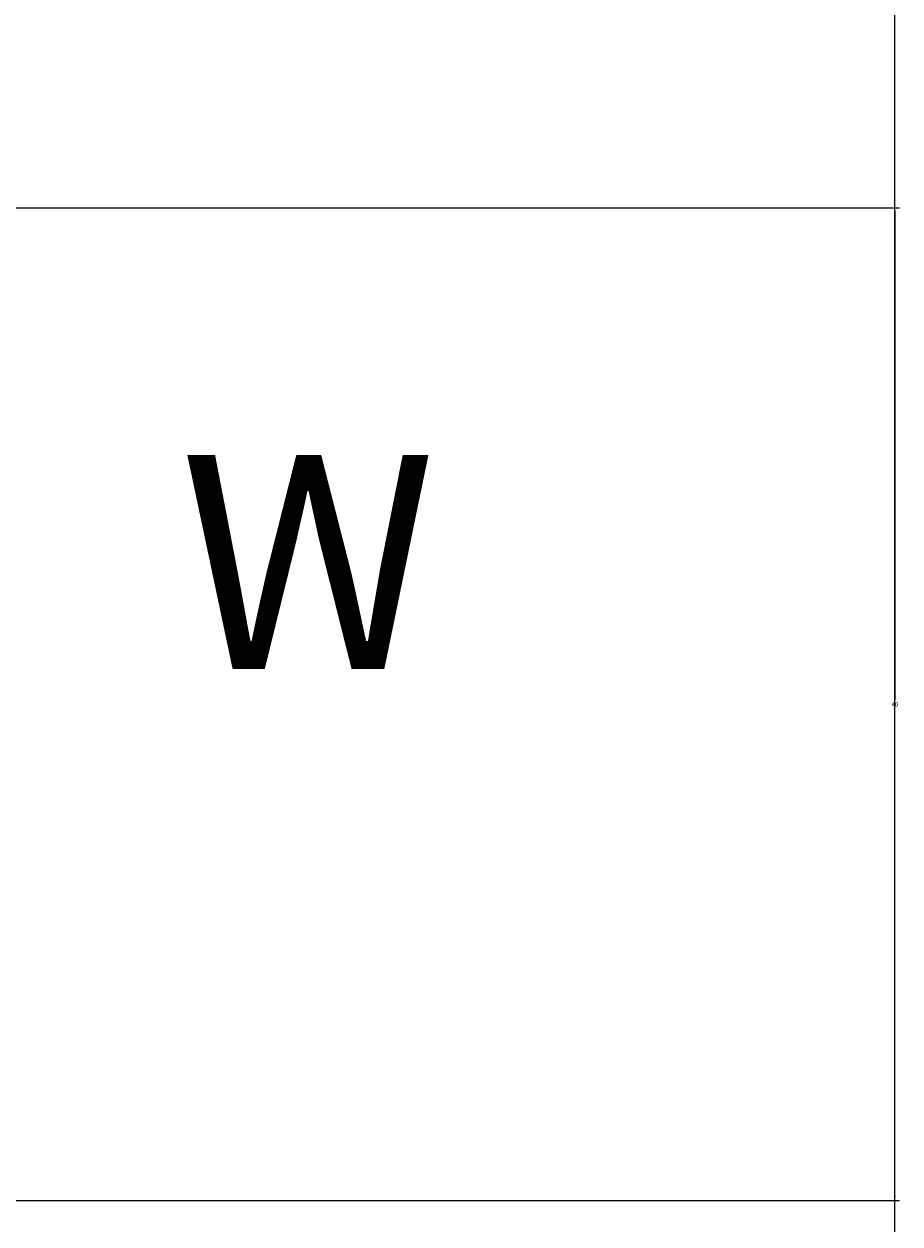
# Model space of a CAD drawing. Units: inches. Extents: x 1568 to 2529, y 2149 to 2897.
# Tile 12 of 16: x 1974 to 2010, y 2410 to 2459. Entities that reach past the tile are written whole.
import ezdxf

# ---------------------------------------------------------------- set-up
doc = ezdxf.new("R2010")
doc.units = ezdxf.units.IN
doc.layers.add('A-ANNO-DIMS', color=2, linetype='Continuous', lineweight=18)
doc.layers.add('text', color=210, linetype='Continuous', lineweight=18)
doc.styles.get("Standard").update_dxf_attribs({"font": 'arial.ttf'})
doc.dimstyles.get("Standard").update_dxf_attribs({"dimtxt": 0.18, "dimasz": 0.18, "dimexe": 0.18, "dimexo": 0.0625, "dimgap": 0.09, "dimtad": 0, "dimtih": 1, "dimtoh": 1, "dimdec": 4, "dimzin": 0, "dimdsep": 46, "dimtxsty": 'Standard', "dimcen": 0.09, "dimadec": 0, "dimazin": 0, "dimtfac": 1, "dimtdec": 4, "dimtofl": 0, "dimtmove": 0, "dimatfit": 3, "dimfxl": 1, "dimtolj": 1, "dimtzin": 0, "dimarcsym": 0})

# ---------------------------------------------------------------- blocks, each defined once
blk = doc.blocks.new('*D28')
at = {"layer": 'A-ANNO-DIMS', "color": 0, "lineweight": -2, "transparency": 16777216}
for p, q in [((1973.643, 2801.532), (2009.61, 2801.532)), ((2009.43, 2801.352), (2009.43, 2501.714)), ((2009.43, 2201.712), (2009.43, 2501.35)), ((1973.613, 2201.532), (2009.61, 2201.532))]:
    blk.add_line(p, q, dxfattribs=at)
at = {"layer": 'A-ANNO-DIMS', "color": 0, "transparency": 16777216}
for points in [[(2009.4, 2801.352), (2009.46, 2801.352), (2009.43, 2801.532)], [(2009.4, 2201.712), (2009.46, 2201.712), (2009.43, 2201.532)]]:
    blk.add_solid(points, dxfattribs=at)
at = {"layer": 'Defpoints', "color": 0, "transparency": 16777216}
for p in [(1973.58, 2801.532), (2009.43, 2801.532), (1973.551, 2201.532)]:
    blk.add_point(p, dxfattribs=at)
at = {"layer": 'A-ANNO-DIMS', "color": 0, "transparency": 16777216, "insert": (2009.43, 2501.532), "char_height": 0.18, "attachment_point": 5}
blk.add_mtext('\\A1;600', dxfattribs=at)
blk = doc.blocks.new('*D35')
at = {"layer": 'A-ANNO-DIMS', "color": 0, "lineweight": -2, "transparency": 16777216}
for p, q in [((1759.113, 2451.227), (2009.61, 2451.227)), ((2009.43, 2451.047), (2009.43, 2431.409)), ((2009.43, 2411.407), (2009.43, 2431.045)), ((1759.113, 2411.227), (2009.61, 2411.227))]:
    blk.add_line(p, q, dxfattribs=at)
at = {"layer": 'A-ANNO-DIMS', "color": 0, "transparency": 16777216}
for points in [[(2009.4, 2451.047), (2009.46, 2451.047), (2009.43, 2451.227)], [(2009.4, 2411.407), (2009.46, 2411.407), (2009.43, 2411.227)]]:
    blk.add_solid(points, dxfattribs=at)
at = {"layer": 'Defpoints', "color": 0, "transparency": 16777216}
for p in [(1759.051, 2451.227), (2009.43, 2451.227), (1759.051, 2411.227)]:
    blk.add_point(p, dxfattribs=at)
at = {"layer": 'A-ANNO-DIMS', "color": 0, "transparency": 16777216, "insert": (2009.43, 2431.227), "char_height": 0.18, "attachment_point": 5}
blk.add_mtext('\\A1;40', dxfattribs=at)

msp = doc.modelspace()

# ---------------------------------------------------------------- texts
at = {"layer": 'text', "insert": (1980.6269, 2441.2738), "char_height": 8.6281, "attachment_point": 1}
msp.add_mtext_dynamic_manual_height_columns('W', width=94.297369, gutter_width=43.1407, heights=[23.0437], dxfattribs=at)

# ---------------------------------------------------------------- dimensions: what is measured, and where the dimension line sits
at = {"layer": 'A-ANNO-DIMS'}
for base, p1, p2, picture, middle in [((2009.4302, 2801.532), (1973.5509, 2201.532), (1973.5802, 2801.532), '*D28', (2009.4302, 2501.532)), ((2009.4302, 2451.2271), (1759.0509, 2411.2271), (1759.0509, 2451.2271), '*D35', (2009.4302, 2431.2271))]:
    dim = msp.add_linear_dim(base=base, p1=p1, p2=p2, angle=90, dimstyle='Standard', override={"dimdec": 0, "dimlfac": 1, "dimrnd": 0, "dimzin": 0, "dimdsep": 46, "dimlunit": 2}, dxfattribs=at)
    dim.commit()
    dim.dimension.update_dxf_attribs({"geometry": picture, "text_midpoint": middle})

doc.saveas('drawing.dxf')
